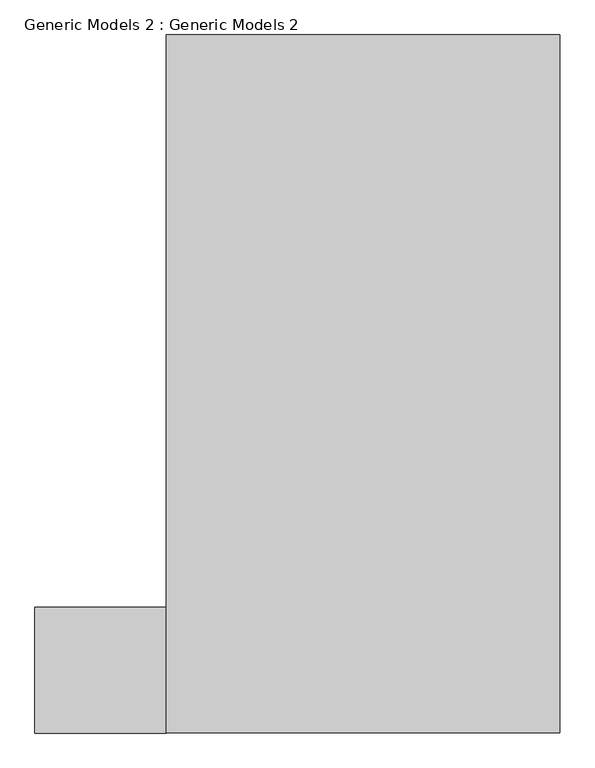
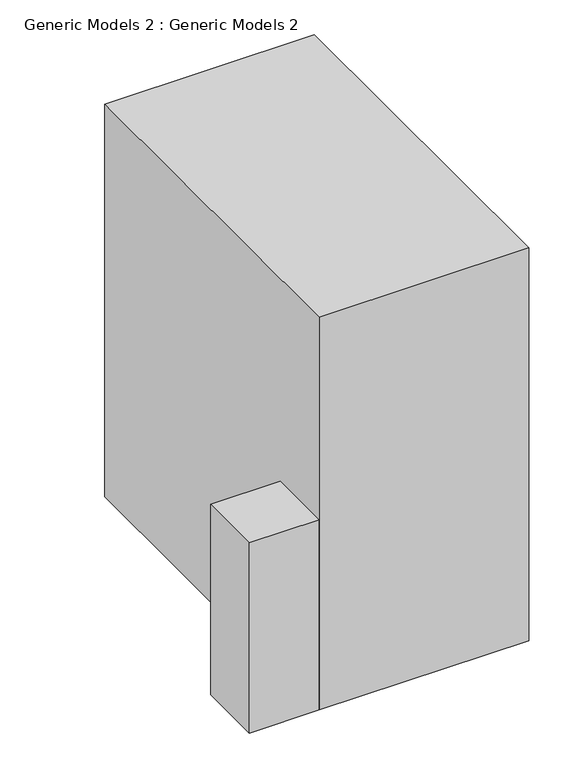
"""IFC4 building model written with IfcOpenShell, lengths in millimetres: proxy geometry, Generic Models 2 : Generic Models 2."""

from ifc_helpers import new_model, si_unit, frame, origin, place, context, project, spatial, polyline, outline, extrude, source, transform, mapped, element, save


def generic_models_2_generic_models_2_10608999(model_context):
    return source(origin(), model_context, "Body", "SweptSolid", [
        extrude(outline(polyline([(-6823.9120831, -7045.9945627), (-6823.9120831, -6131.5945627), (-5871.4120831, -6131.5945627), (-5871.4120831, -7045.9945627), (-6823.9120831, -7045.9945627)])), frame((0.0, 0.0, 3352.8), z_axis=(0.0, 0.0, 1.0), x_axis=(1.0, 0.0, 0.0)), (0.0, 0.0, 1.0), 2743.2),
        extrude(outline(polyline([(-3013.9120831, -1978.6945627), (-3013.9120831, -7045.9945627), (-5871.4120831, -7045.9945627), (-5871.4120831, -1978.6945627), (-3013.9120831, -1978.6945627)])), frame((0.0, 0.0, 3352.8), z_axis=(0.0, 0.0, 1.0), x_axis=(1.0, 0.0, 0.0)), (0.0, 0.0, 1.0), 5662.5547159),
    ])


if __name__ == "__main__":
    model = new_model("IFC4")
    model_context = context("Model", 3, world=origin())
    ifc_project = project(units=[si_unit("LENGTHUNIT", "METRE", prefix="MILLI")], contexts=[model_context])
    site = spatial("IfcSite", under=ifc_project)
    building = spatial("IfcBuilding", under=site)
    placement = place(None, origin())
    generic_models_2_generic_models_2_shape = generic_models_2_generic_models_2_10608999(model_context)
    element("IfcBuildingElementProxy", 1, Name="Generic Models 2 : Generic Models 2", ObjectType="Generic Models 2 : Generic Models 2", at=placement, inside=building, context=model_context, shape_type="MappedRepresentation", body=[
        mapped(generic_models_2_generic_models_2_shape, transform((0.0, 0.0, 0.0), x_axis=(1.0, 0.0, 0.0), y_axis=(0.0, 1.0, 0.0), z_axis=(0.0, 0.0, 1.0))),
    ])
    save(model, "model.ifc")
